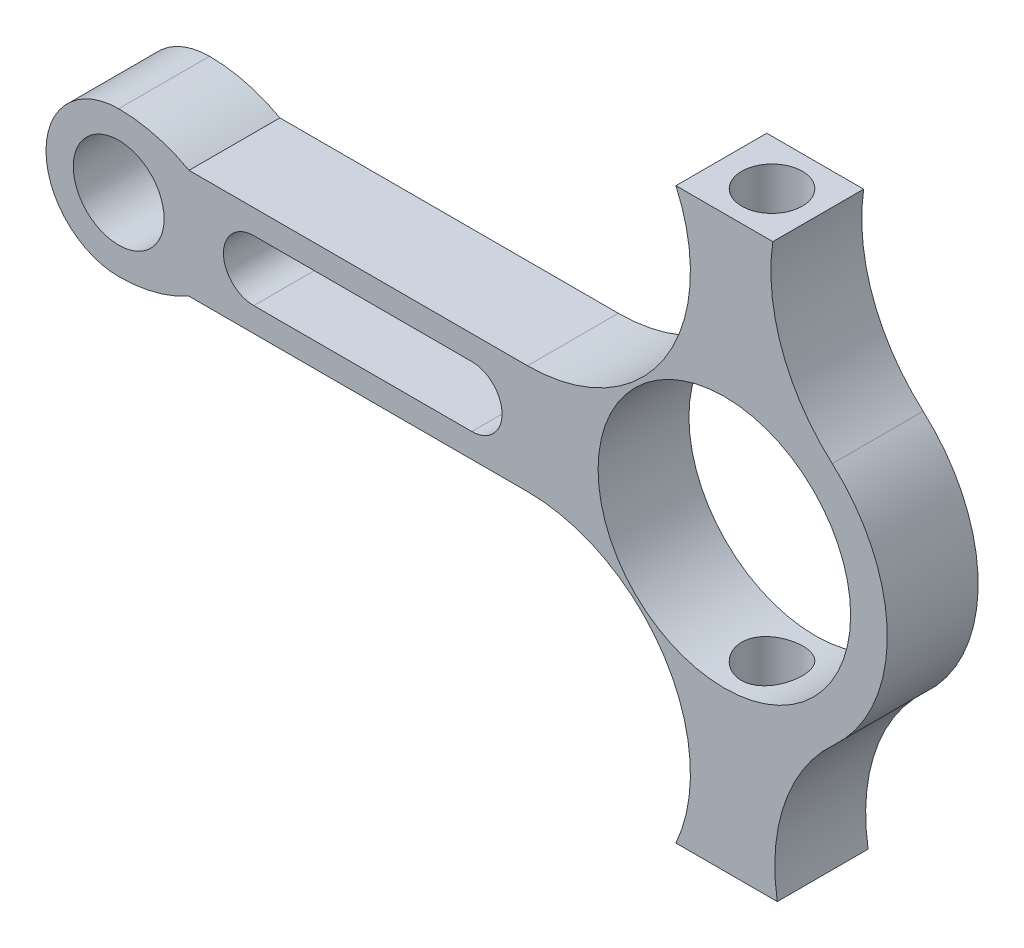
ISO-10303-21;
HEADER;
FILE_DESCRIPTION(('STEP AP214'),'2;1');
FILE_NAME('part.step','',(''),(''),'','','');
FILE_SCHEMA(('AUTOMOTIVE_DESIGN { 1 0 10303 214 1 1 1 1 }'));
ENDSEC;
DATA;
#1=APPLICATION_CONTEXT('core data for automotive mechanical design processes');
#2=APPLICATION_PROTOCOL_DEFINITION('international standard','automotive_design',2000,#1);
#3=PRODUCT_CONTEXT('',#1,'mechanical');
#4=PRODUCT('Part','Part','',(#3));
#5=PRODUCT_RELATED_PRODUCT_CATEGORY('part','',(#4));
#6=PRODUCT_DEFINITION_FORMATION('','',#4);
#7=PRODUCT_DEFINITION_CONTEXT('part definition',#1,'design');
#8=PRODUCT_DEFINITION('design','',#6,#7);
#9=PRODUCT_DEFINITION_SHAPE('','',#8);
#10=(LENGTH_UNIT() NAMED_UNIT(*) SI_UNIT(.MILLI.,.METRE.));
#11=(NAMED_UNIT(*) PLANE_ANGLE_UNIT() SI_UNIT($,.RADIAN.));
#12=(NAMED_UNIT(*) SI_UNIT($,.STERADIAN.) SOLID_ANGLE_UNIT());
#13=UNCERTAINTY_MEASURE_WITH_UNIT(LENGTH_MEASURE(1.E-05),#10,'distance_accuracy_value','');
#14=(GEOMETRIC_REPRESENTATION_CONTEXT(3) GLOBAL_UNCERTAINTY_ASSIGNED_CONTEXT((#13)) GLOBAL_UNIT_ASSIGNED_CONTEXT((#10,
#11,#12)) REPRESENTATION_CONTEXT('',''));
#15=CARTESIAN_POINT('',(0.,0.,0.));
#16=DIRECTION('',(0.,0.,1.));
#17=DIRECTION('',(1.,0.,0.));
#18=AXIS2_PLACEMENT_3D('',#15,#16,#17);
#19=CARTESIAN_POINT('',(137.680790343127,42.6352910054251,15.));
#20=DIRECTION('',(0.,0.,1.));
#21=DIRECTION('',(1.,0.,0.));
#22=AXIS2_PLACEMENT_3D('',#19,#20,#21);
#23=PLANE('',#22);
#24=CARTESIAN_POINT('',(0.,0.,15.));
#25=DIRECTION('',(0.,0.,1.));
#26=DIRECTION('',(1.,0.,0.));
#27=AXIS2_PLACEMENT_3D('',#24,#25,#26);
#28=CIRCLE('',#27,7.5);
#29=CARTESIAN_POINT('',(7.5,0.,15.));
#30=VERTEX_POINT('',#29);
#31=EDGE_CURVE('E208',#30,#30,#28,.T.);
#32=ORIENTED_EDGE('',*,*,#31,.F.);
#33=EDGE_LOOP('',(#32));
#34=FACE_BOUND('',#33,.T.);
#35=DIRECTION('',(-1.,0.,0.));
#36=VECTOR('',#35,1.);
#37=CARTESIAN_POINT('',(100.,47.,15.));
#38=LINE('',#37,#36);
#39=CARTESIAN_POINT('',(108.,47.,15.));
#40=VERTEX_POINT('',#39);
#41=CARTESIAN_POINT('',(92.,47.,15.));
#42=VERTEX_POINT('',#41);
#43=EDGE_CURVE('E212',#40,#42,#38,.T.);
#44=ORIENTED_EDGE('',*,*,#43,.T.);
#45=CARTESIAN_POINT('',(67.4969389667332,35.9,15.));
#46=DIRECTION('',(0.,0.,-1.));
#47=DIRECTION('',(-1.,0.,0.));
#48=AXIS2_PLACEMENT_3D('',#45,#46,#47);
#49=CIRCLE('',#48,26.9);
#50=CARTESIAN_POINT('',(67.4969389667332,9.,15.));
#51=VERTEX_POINT('',#50);
#52=EDGE_CURVE('E216',#42,#51,#49,.T.);
#53=ORIENTED_EDGE('',*,*,#52,.T.);
#54=DIRECTION('',(-1.,0.,0.));
#55=VECTOR('',#54,1.);
#56=CARTESIAN_POINT('',(11.6189500386222,9.,15.));
#57=LINE('',#56,#55);
#58=CARTESIAN_POINT('',(11.6189500386222,9.,15.));
#59=VERTEX_POINT('',#58);
#60=EDGE_CURVE('E218',#51,#59,#57,.T.);
#61=ORIENTED_EDGE('',*,*,#60,.T.);
#62=CARTESIAN_POINT('',(0.,-12.,15.));
#63=DIRECTION('',(0.,0.,1.));
#64=DIRECTION('',(-1.,0.,0.));
#65=AXIS2_PLACEMENT_3D('',#62,#63,#64);
#66=CIRCLE('',#65,24.);
#67=CARTESIAN_POINT('',(0.,12.,15.));
#68=VERTEX_POINT('',#67);
#69=EDGE_CURVE('E222',#59,#68,#66,.T.);
#70=ORIENTED_EDGE('',*,*,#69,.T.);
#71=CARTESIAN_POINT('',(0.,0.,15.));
#72=DIRECTION('',(0.,0.,1.));
#73=DIRECTION('',(1.,0.,0.));
#74=AXIS2_PLACEMENT_3D('',#71,#72,#73);
#75=CIRCLE('',#74,12.);
#76=CARTESIAN_POINT('',(0.,-12.,15.));
#77=VERTEX_POINT('',#76);
#78=EDGE_CURVE('E224',#68,#77,#75,.T.);
#79=ORIENTED_EDGE('',*,*,#78,.T.);
#80=CARTESIAN_POINT('',(0.,12.,15.));
#81=DIRECTION('',(0.,0.,1.));
#82=DIRECTION('',(1.,0.,0.));
#83=AXIS2_PLACEMENT_3D('',#80,#81,#82);
#84=CIRCLE('',#83,24.);
#85=CARTESIAN_POINT('',(11.6189500386223,-9.,15.));
#86=VERTEX_POINT('',#85);
#87=EDGE_CURVE('E223',#77,#86,#84,.T.);
#88=ORIENTED_EDGE('',*,*,#87,.T.);
#89=DIRECTION('',(1.,0.,0.));
#90=VECTOR('',#89,1.);
#91=CARTESIAN_POINT('',(11.6189500386223,-9.,15.));
#92=LINE('',#91,#90);
#93=CARTESIAN_POINT('',(67.4969389667332,-8.99999999999999,15.));
#94=VERTEX_POINT('',#93);
#95=EDGE_CURVE('E226',#86,#94,#92,.T.);
#96=ORIENTED_EDGE('',*,*,#95,.T.);
#97=CARTESIAN_POINT('',(67.4969389667332,-35.9,15.));
#98=DIRECTION('',(0.,0.,-1.));
#99=DIRECTION('',(1.,0.,0.));
#100=AXIS2_PLACEMENT_3D('',#97,#98,#99);
#101=CIRCLE('',#100,26.9);
#102=CARTESIAN_POINT('',(92.,-47.,15.));
#103=VERTEX_POINT('',#102);
#104=EDGE_CURVE('E228',#94,#103,#101,.T.);
#105=ORIENTED_EDGE('',*,*,#104,.T.);
#106=DIRECTION('',(1.,0.,0.));
#107=VECTOR('',#106,1.);
#108=CARTESIAN_POINT('',(100.,-47.,15.));
#109=LINE('',#108,#107);
#110=CARTESIAN_POINT('',(108.73655717955,-47.,15.));
#111=VERTEX_POINT('',#110);
#112=EDGE_CURVE('E233',#103,#111,#109,.T.);
#113=ORIENTED_EDGE('',*,*,#112,.T.);
#114=CARTESIAN_POINT('',(138.32635427095,-42.0559219171047,15.));
#115=DIRECTION('',(0.,0.,-1.));
#116=DIRECTION('',(-1.,0.,0.));
#117=AXIS2_PLACEMENT_3D('',#114,#115,#116);
#118=CIRCLE('',#117,30.);
#119=CARTESIAN_POINT('',(118.119137607883,-19.8823251242551,15.));
#120=VERTEX_POINT('',#119);
#121=EDGE_CURVE('E231',#111,#120,#118,.T.);
#122=ORIENTED_EDGE('',*,*,#121,.T.);
#123=CARTESIAN_POINT('',(100.,0.,15.));
#124=DIRECTION('',(0.,0.,1.));
#125=DIRECTION('',(1.,0.,0.));
#126=AXIS2_PLACEMENT_3D('',#123,#124,#125);
#127=CIRCLE('',#126,26.9);
#128=CARTESIAN_POINT('',(117.813941304572,20.1562272064312,15.));
#129=VERTEX_POINT('',#128);
#130=EDGE_CURVE('E234',#120,#129,#127,.T.);
#131=ORIENTED_EDGE('',*,*,#130,.T.);
#132=CARTESIAN_POINT('',(137.680790343127,42.6352910054251,15.));
#133=DIRECTION('',(0.,0.,-1.));
#134=DIRECTION('',(1.,0.,0.));
#135=AXIS2_PLACEMENT_3D('',#132,#133,#134);
#136=CIRCLE('',#135,30.);
#137=EDGE_CURVE('E240',#129,#40,#136,.T.);
#138=ORIENTED_EDGE('',*,*,#137,.T.);
#139=EDGE_LOOP('',(#44,#53,#61,#70,#79,#88,#96,#105,#113,#122,#131,#138));
#140=FACE_BOUND('',#139,.T.);
#141=CARTESIAN_POINT('',(100.,0.,15.));
#142=DIRECTION('',(0.,0.,1.));
#143=DIRECTION('',(1.,0.,0.));
#144=AXIS2_PLACEMENT_3D('',#141,#142,#143);
#145=CIRCLE('',#144,20.85);
#146=CARTESIAN_POINT('',(120.85,0.,15.));
#147=VERTEX_POINT('',#146);
#148=EDGE_CURVE('E205',#147,#147,#145,.T.);
#149=ORIENTED_EDGE('',*,*,#148,.F.);
#150=EDGE_LOOP('',(#149));
#151=FACE_BOUND('',#150,.T.);
#152=DIRECTION('',(1.,0.,0.));
#153=VECTOR('',#152,1.);
#154=CARTESIAN_POINT('',(22.3,-5.,15.));
#155=LINE('',#154,#153);
#156=CARTESIAN_POINT('',(22.3,-5.,15.));
#157=VERTEX_POINT('',#156);
#158=CARTESIAN_POINT('',(58.3,-5.,15.));
#159=VERTEX_POINT('',#158);
#160=EDGE_CURVE('E175',#157,#159,#155,.T.);
#161=ORIENTED_EDGE('',*,*,#160,.F.);
#162=CARTESIAN_POINT('',(22.3,0.,15.));
#163=DIRECTION('',(0.,0.,1.));
#164=DIRECTION('',(1.,0.,0.));
#165=AXIS2_PLACEMENT_3D('',#162,#163,#164);
#166=CIRCLE('',#165,5.);
#167=CARTESIAN_POINT('',(22.3,5.,15.));
#168=VERTEX_POINT('',#167);
#169=EDGE_CURVE('E164',#168,#157,#166,.T.);
#170=ORIENTED_EDGE('',*,*,#169,.F.);
#171=DIRECTION('',(-1.,0.,0.));
#172=VECTOR('',#171,1.);
#173=CARTESIAN_POINT('',(22.3,5.,15.));
#174=LINE('',#173,#172);
#175=CARTESIAN_POINT('',(58.3,5.,15.));
#176=VERTEX_POINT('',#175);
#177=EDGE_CURVE('E186',#176,#168,#174,.T.);
#178=ORIENTED_EDGE('',*,*,#177,.F.);
#179=CARTESIAN_POINT('',(58.3,0.,15.));
#180=DIRECTION('',(0.,0.,1.));
#181=DIRECTION('',(1.,0.,0.));
#182=AXIS2_PLACEMENT_3D('',#179,#180,#181);
#183=CIRCLE('',#182,5.);
#184=EDGE_CURVE('E183',#159,#176,#183,.T.);
#185=ORIENTED_EDGE('',*,*,#184,.F.);
#186=EDGE_LOOP('',(#161,#170,#178,#185));
#187=FACE_BOUND('',#186,.T.);
#188=ADVANCED_FACE('F44',(#34,#140,#151,#187),#23,.T.);
#189=CARTESIAN_POINT('',(137.680790343127,42.6352910054251,0.));
#190=DIRECTION('',(0.,0.,1.));
#191=DIRECTION('',(1.,0.,0.));
#192=AXIS2_PLACEMENT_3D('',#189,#190,#191);
#193=PLANE('',#192);
#194=CARTESIAN_POINT('',(100.,0.,0.));
#195=DIRECTION('',(0.,0.,1.));
#196=DIRECTION('',(1.,0.,0.));
#197=AXIS2_PLACEMENT_3D('',#194,#195,#196);
#198=CIRCLE('',#197,20.85);
#199=CARTESIAN_POINT('',(120.85,0.,0.));
#200=VERTEX_POINT('',#199);
#201=EDGE_CURVE('E182',#200,#200,#198,.T.);
#202=ORIENTED_EDGE('',*,*,#201,.T.);
#203=EDGE_LOOP('',(#202));
#204=FACE_BOUND('',#203,.T.);
#205=CARTESIAN_POINT('',(0.,0.,0.));
#206=DIRECTION('',(0.,0.,1.));
#207=DIRECTION('',(1.,0.,0.));
#208=AXIS2_PLACEMENT_3D('',#205,#206,#207);
#209=CIRCLE('',#208,7.5);
#210=CARTESIAN_POINT('',(7.5,0.,0.));
#211=VERTEX_POINT('',#210);
#212=EDGE_CURVE('E202',#211,#211,#209,.T.);
#213=ORIENTED_EDGE('',*,*,#212,.T.);
#214=EDGE_LOOP('',(#213));
#215=FACE_BOUND('',#214,.T.);
#216=DIRECTION('',(-1.,0.,0.));
#217=VECTOR('',#216,1.);
#218=CARTESIAN_POINT('',(100.,47.,0.));
#219=LINE('',#218,#217);
#220=CARTESIAN_POINT('',(108.,47.,0.));
#221=VERTEX_POINT('',#220);
#222=CARTESIAN_POINT('',(92.,47.,0.));
#223=VERTEX_POINT('',#222);
#224=EDGE_CURVE('E211',#221,#223,#219,.T.);
#225=ORIENTED_EDGE('',*,*,#224,.F.);
#226=CARTESIAN_POINT('',(137.680790343127,42.6352910054251,0.));
#227=DIRECTION('',(0.,0.,-1.));
#228=DIRECTION('',(1.,0.,0.));
#229=AXIS2_PLACEMENT_3D('',#226,#227,#228);
#230=CIRCLE('',#229,30.);
#231=CARTESIAN_POINT('',(117.813941304572,20.1562272064312,0.));
#232=VERTEX_POINT('',#231);
#233=EDGE_CURVE('E220',#232,#221,#230,.T.);
#234=ORIENTED_EDGE('',*,*,#233,.F.);
#235=CARTESIAN_POINT('',(100.,0.,0.));
#236=DIRECTION('',(0.,0.,1.));
#237=DIRECTION('',(1.,0.,0.));
#238=AXIS2_PLACEMENT_3D('',#235,#236,#237);
#239=CIRCLE('',#238,26.9);
#240=CARTESIAN_POINT('',(118.119137607883,-19.8823251242551,0.));
#241=VERTEX_POINT('',#240);
#242=EDGE_CURVE('E257',#241,#232,#239,.T.);
#243=ORIENTED_EDGE('',*,*,#242,.F.);
#244=CARTESIAN_POINT('',(138.32635427095,-42.0559219171047,0.));
#245=DIRECTION('',(0.,0.,-1.));
#246=DIRECTION('',(-1.,0.,0.));
#247=AXIS2_PLACEMENT_3D('',#244,#245,#246);
#248=CIRCLE('',#247,30.);
#249=CARTESIAN_POINT('',(108.73655717955,-47.,0.));
#250=VERTEX_POINT('',#249);
#251=EDGE_CURVE('E256',#250,#241,#248,.T.);
#252=ORIENTED_EDGE('',*,*,#251,.F.);
#253=DIRECTION('',(1.,0.,0.));
#254=VECTOR('',#253,1.);
#255=CARTESIAN_POINT('',(100.,-47.,0.));
#256=LINE('',#255,#254);
#257=CARTESIAN_POINT('',(92.,-47.,0.));
#258=VERTEX_POINT('',#257);
#259=EDGE_CURVE('E258',#258,#250,#256,.T.);
#260=ORIENTED_EDGE('',*,*,#259,.F.);
#261=CARTESIAN_POINT('',(67.4969389667332,-35.9,0.));
#262=DIRECTION('',(0.,0.,-1.));
#263=DIRECTION('',(1.,0.,0.));
#264=AXIS2_PLACEMENT_3D('',#261,#262,#263);
#265=CIRCLE('',#264,26.9);
#266=CARTESIAN_POINT('',(67.4969389667332,-8.99999999999999,0.));
#267=VERTEX_POINT('',#266);
#268=EDGE_CURVE('E251',#267,#258,#265,.T.);
#269=ORIENTED_EDGE('',*,*,#268,.F.);
#270=DIRECTION('',(1.,0.,0.));
#271=VECTOR('',#270,1.);
#272=CARTESIAN_POINT('',(11.6189500386223,-9.,0.));
#273=LINE('',#272,#271);
#274=CARTESIAN_POINT('',(11.6189500386223,-9.,0.));
#275=VERTEX_POINT('',#274);
#276=EDGE_CURVE('E253',#275,#267,#273,.T.);
#277=ORIENTED_EDGE('',*,*,#276,.F.);
#278=CARTESIAN_POINT('',(0.,12.,0.));
#279=DIRECTION('',(0.,0.,1.));
#280=DIRECTION('',(1.,0.,0.));
#281=AXIS2_PLACEMENT_3D('',#278,#279,#280);
#282=CIRCLE('',#281,24.);
#283=CARTESIAN_POINT('',(0.,-12.,0.));
#284=VERTEX_POINT('',#283);
#285=EDGE_CURVE('E247',#284,#275,#282,.T.);
#286=ORIENTED_EDGE('',*,*,#285,.F.);
#287=CARTESIAN_POINT('',(0.,0.,0.));
#288=DIRECTION('',(0.,0.,1.));
#289=DIRECTION('',(1.,0.,0.));
#290=AXIS2_PLACEMENT_3D('',#287,#288,#289);
#291=CIRCLE('',#290,12.);
#292=CARTESIAN_POINT('',(0.,12.,0.));
#293=VERTEX_POINT('',#292);
#294=EDGE_CURVE('E250',#293,#284,#291,.T.);
#295=ORIENTED_EDGE('',*,*,#294,.F.);
#296=CARTESIAN_POINT('',(0.,-12.,0.));
#297=DIRECTION('',(0.,0.,1.));
#298=DIRECTION('',(-1.,0.,0.));
#299=AXIS2_PLACEMENT_3D('',#296,#297,#298);
#300=CIRCLE('',#299,24.);
#301=CARTESIAN_POINT('',(11.6189500386222,9.,0.));
#302=VERTEX_POINT('',#301);
#303=EDGE_CURVE('E242',#302,#293,#300,.T.);
#304=ORIENTED_EDGE('',*,*,#303,.F.);
#305=DIRECTION('',(-1.,0.,0.));
#306=VECTOR('',#305,1.);
#307=CARTESIAN_POINT('',(11.6189500386222,9.,0.));
#308=LINE('',#307,#306);
#309=CARTESIAN_POINT('',(67.4969389667332,9.,0.));
#310=VERTEX_POINT('',#309);
#311=EDGE_CURVE('E245',#310,#302,#308,.T.);
#312=ORIENTED_EDGE('',*,*,#311,.F.);
#313=CARTESIAN_POINT('',(67.4969389667332,35.9,0.));
#314=DIRECTION('',(0.,0.,-1.));
#315=DIRECTION('',(-1.,0.,0.));
#316=AXIS2_PLACEMENT_3D('',#313,#314,#315);
#317=CIRCLE('',#316,26.9);
#318=EDGE_CURVE('E244',#223,#310,#317,.T.);
#319=ORIENTED_EDGE('',*,*,#318,.F.);
#320=EDGE_LOOP('',(#225,#234,#243,#252,#260,#269,#277,#286,#295,#304,#312,#319));
#321=FACE_BOUND('',#320,.T.);
#322=CARTESIAN_POINT('',(22.3,0.,0.));
#323=DIRECTION('',(0.,0.,1.));
#324=DIRECTION('',(1.,0.,0.));
#325=AXIS2_PLACEMENT_3D('',#322,#323,#324);
#326=CIRCLE('',#325,5.);
#327=CARTESIAN_POINT('',(22.3,5.,0.));
#328=VERTEX_POINT('',#327);
#329=CARTESIAN_POINT('',(22.3,-5.,0.));
#330=VERTEX_POINT('',#329);
#331=EDGE_CURVE('E73',#328,#330,#326,.T.);
#332=ORIENTED_EDGE('',*,*,#331,.T.);
#333=DIRECTION('',(1.,0.,0.));
#334=VECTOR('',#333,1.);
#335=CARTESIAN_POINT('',(22.3,-5.,0.));
#336=LINE('',#335,#334);
#337=CARTESIAN_POINT('',(58.3,-5.,0.));
#338=VERTEX_POINT('',#337);
#339=EDGE_CURVE('E179',#330,#338,#336,.T.);
#340=ORIENTED_EDGE('',*,*,#339,.T.);
#341=CARTESIAN_POINT('',(58.3,0.,0.));
#342=DIRECTION('',(0.,0.,1.));
#343=DIRECTION('',(1.,0.,0.));
#344=AXIS2_PLACEMENT_3D('',#341,#342,#343);
#345=CIRCLE('',#344,5.);
#346=CARTESIAN_POINT('',(58.3,5.,0.));
#347=VERTEX_POINT('',#346);
#348=EDGE_CURVE('E192',#338,#347,#345,.T.);
#349=ORIENTED_EDGE('',*,*,#348,.T.);
#350=DIRECTION('',(-1.,0.,0.));
#351=VECTOR('',#350,1.);
#352=CARTESIAN_POINT('',(22.3,5.,0.));
#353=LINE('',#352,#351);
#354=EDGE_CURVE('E173',#347,#328,#353,.T.);
#355=ORIENTED_EDGE('',*,*,#354,.T.);
#356=EDGE_LOOP('',(#332,#340,#349,#355));
#357=FACE_BOUND('',#356,.T.);
#358=ADVANCED_FACE('F326',(#204,#215,#321,#357),#193,.F.);
#359=CARTESIAN_POINT('',(100.,47.,15.));
#360=DIRECTION('',(0.,-1.,0.));
#361=DIRECTION('',(0.,0.,-1.));
#362=AXIS2_PLACEMENT_3D('',#359,#360,#361);
#363=PLANE('',#362);
#364=CARTESIAN_POINT('',(100.368278589775,47.,7.5));
#365=DIRECTION('',(0.,-1.,0.));
#366=DIRECTION('',(0.,0.,-1.));
#367=AXIS2_PLACEMENT_3D('',#364,#365,#366);
#368=CIRCLE('',#367,5.);
#369=CARTESIAN_POINT('',(100.368278589775,47.,2.5));
#370=VERTEX_POINT('',#369);
#371=EDGE_CURVE('E298',#370,#370,#368,.T.);
#372=ORIENTED_EDGE('',*,*,#371,.T.);
#373=EDGE_LOOP('',(#372));
#374=FACE_BOUND('',#373,.T.);
#375=ORIENTED_EDGE('',*,*,#224,.T.);
#376=DIRECTION('',(0.,0.,-1.));
#377=VECTOR('',#376,1.);
#378=CARTESIAN_POINT('',(92.,47.,15.));
#379=LINE('',#378,#377);
#380=EDGE_CURVE('E11',#42,#223,#379,.T.);
#381=ORIENTED_EDGE('',*,*,#380,.F.);
#382=ORIENTED_EDGE('',*,*,#43,.F.);
#383=DIRECTION('',(0.,0.,-1.));
#384=VECTOR('',#383,1.);
#385=CARTESIAN_POINT('',(108.,47.,15.));
#386=LINE('',#385,#384);
#387=EDGE_CURVE('E239',#40,#221,#386,.T.);
#388=ORIENTED_EDGE('',*,*,#387,.T.);
#389=EDGE_LOOP('',(#375,#381,#382,#388));
#390=FACE_BOUND('',#389,.T.);
#391=ADVANCED_FACE('F50',(#374,#390),#363,.F.);
#392=CARTESIAN_POINT('',(67.4969389667332,35.9,15.));
#393=DIRECTION('',(0.,0.,-1.));
#394=DIRECTION('',(-1.,0.,0.));
#395=AXIS2_PLACEMENT_3D('',#392,#393,#394);
#396=CYLINDRICAL_SURFACE('',#395,26.9);
#397=ORIENTED_EDGE('',*,*,#318,.T.);
#398=DIRECTION('',(0.,0.,-1.));
#399=VECTOR('',#398,1.);
#400=CARTESIAN_POINT('',(67.4969389667332,9.,15.));
#401=LINE('',#400,#399);
#402=EDGE_CURVE('E56',#51,#310,#401,.T.);
#403=ORIENTED_EDGE('',*,*,#402,.F.);
#404=ORIENTED_EDGE('',*,*,#52,.F.);
#405=ORIENTED_EDGE('',*,*,#380,.T.);
#406=EDGE_LOOP('',(#397,#403,#404,#405));
#407=FACE_BOUND('',#406,.T.);
#408=ADVANCED_FACE('F376',(#407),#396,.F.);
#409=CARTESIAN_POINT('',(11.6189500386222,9.,15.));
#410=DIRECTION('',(0.,-1.,0.));
#411=DIRECTION('',(0.,0.,-1.));
#412=AXIS2_PLACEMENT_3D('',#409,#410,#411);
#413=PLANE('',#412);
#414=ORIENTED_EDGE('',*,*,#311,.T.);
#415=DIRECTION('',(0.,0.,-1.));
#416=VECTOR('',#415,1.);
#417=CARTESIAN_POINT('',(11.6189500386222,9.,15.));
#418=LINE('',#417,#416);
#419=EDGE_CURVE('E289',#59,#302,#418,.T.);
#420=ORIENTED_EDGE('',*,*,#419,.F.);
#421=ORIENTED_EDGE('',*,*,#60,.F.);
#422=ORIENTED_EDGE('',*,*,#402,.T.);
#423=EDGE_LOOP('',(#414,#420,#421,#422));
#424=FACE_BOUND('',#423,.T.);
#425=ADVANCED_FACE('F373',(#424),#413,.F.);
#426=CARTESIAN_POINT('',(0.,-12.,15.));
#427=DIRECTION('',(0.,0.,-1.));
#428=DIRECTION('',(-1.,0.,0.));
#429=AXIS2_PLACEMENT_3D('',#426,#427,#428);
#430=CYLINDRICAL_SURFACE('',#429,24.);
#431=ORIENTED_EDGE('',*,*,#303,.T.);
#432=DIRECTION('',(0.,0.,-1.));
#433=VECTOR('',#432,1.);
#434=CARTESIAN_POINT('',(0.,12.,15.));
#435=LINE('',#434,#433);
#436=EDGE_CURVE('E290',#68,#293,#435,.T.);
#437=ORIENTED_EDGE('',*,*,#436,.F.);
#438=ORIENTED_EDGE('',*,*,#69,.F.);
#439=ORIENTED_EDGE('',*,*,#419,.T.);
#440=EDGE_LOOP('',(#431,#437,#438,#439));
#441=FACE_BOUND('',#440,.T.);
#442=ADVANCED_FACE('F369',(#441),#430,.T.);
#443=CARTESIAN_POINT('',(0.,0.,15.));
#444=DIRECTION('',(0.,0.,-1.));
#445=DIRECTION('',(-1.,0.,0.));
#446=AXIS2_PLACEMENT_3D('',#443,#444,#445);
#447=CYLINDRICAL_SURFACE('',#446,12.);
#448=ORIENTED_EDGE('',*,*,#294,.T.);
#449=DIRECTION('',(0.,0.,-1.));
#450=VECTOR('',#449,1.);
#451=CARTESIAN_POINT('',(0.,-12.,15.));
#452=LINE('',#451,#450);
#453=EDGE_CURVE('E283',#77,#284,#452,.T.);
#454=ORIENTED_EDGE('',*,*,#453,.F.);
#455=ORIENTED_EDGE('',*,*,#78,.F.);
#456=ORIENTED_EDGE('',*,*,#436,.T.);
#457=EDGE_LOOP('',(#448,#454,#455,#456));
#458=FACE_BOUND('',#457,.T.);
#459=ADVANCED_FACE('F364',(#458),#447,.T.);
#460=CARTESIAN_POINT('',(0.,12.,15.));
#461=DIRECTION('',(0.,0.,-1.));
#462=DIRECTION('',(-1.,0.,0.));
#463=AXIS2_PLACEMENT_3D('',#460,#461,#462);
#464=CYLINDRICAL_SURFACE('',#463,24.);
#465=ORIENTED_EDGE('',*,*,#285,.T.);
#466=DIRECTION('',(0.,0.,-1.));
#467=VECTOR('',#466,1.);
#468=CARTESIAN_POINT('',(11.6189500386223,-9.,15.));
#469=LINE('',#468,#467);
#470=EDGE_CURVE('E284',#86,#275,#469,.T.);
#471=ORIENTED_EDGE('',*,*,#470,.F.);
#472=ORIENTED_EDGE('',*,*,#87,.F.);
#473=ORIENTED_EDGE('',*,*,#453,.T.);
#474=EDGE_LOOP('',(#465,#471,#472,#473));
#475=FACE_BOUND('',#474,.T.);
#476=ADVANCED_FACE('F363',(#475),#464,.T.);
#477=CARTESIAN_POINT('',(11.6189500386223,-9.,15.));
#478=DIRECTION('',(0.,1.,0.));
#479=DIRECTION('',(-1.,0.,0.));
#480=AXIS2_PLACEMENT_3D('',#477,#478,#479);
#481=PLANE('',#480);
#482=ORIENTED_EDGE('',*,*,#276,.T.);
#483=DIRECTION('',(0.,0.,-1.));
#484=VECTOR('',#483,1.);
#485=CARTESIAN_POINT('',(67.4969389667332,-8.99999999999999,15.));
#486=LINE('',#485,#484);
#487=EDGE_CURVE('E279',#94,#267,#486,.T.);
#488=ORIENTED_EDGE('',*,*,#487,.F.);
#489=ORIENTED_EDGE('',*,*,#95,.F.);
#490=ORIENTED_EDGE('',*,*,#470,.T.);
#491=EDGE_LOOP('',(#482,#488,#489,#490));
#492=FACE_BOUND('',#491,.T.);
#493=ADVANCED_FACE('F360',(#492),#481,.F.);
#494=CARTESIAN_POINT('',(67.4969389667332,-35.9,15.));
#495=DIRECTION('',(0.,0.,-1.));
#496=DIRECTION('',(-1.,0.,0.));
#497=AXIS2_PLACEMENT_3D('',#494,#495,#496);
#498=CYLINDRICAL_SURFACE('',#497,26.9);
#499=ORIENTED_EDGE('',*,*,#268,.T.);
#500=DIRECTION('',(0.,0.,-1.));
#501=VECTOR('',#500,1.);
#502=CARTESIAN_POINT('',(92.,-47.,15.));
#503=LINE('',#502,#501);
#504=EDGE_CURVE('E274',#103,#258,#503,.T.);
#505=ORIENTED_EDGE('',*,*,#504,.F.);
#506=ORIENTED_EDGE('',*,*,#104,.F.);
#507=ORIENTED_EDGE('',*,*,#487,.T.);
#508=EDGE_LOOP('',(#499,#505,#506,#507));
#509=FACE_BOUND('',#508,.T.);
#510=ADVANCED_FACE('F355',(#509),#498,.F.);
#511=CARTESIAN_POINT('',(100.,-47.,15.));
#512=DIRECTION('',(0.,1.,0.));
#513=DIRECTION('',(0.,0.,1.));
#514=AXIS2_PLACEMENT_3D('',#511,#512,#513);
#515=PLANE('',#514);
#516=CARTESIAN_POINT('',(100.368278589775,-47.,7.5));
#517=DIRECTION('',(0.,-1.,0.));
#518=DIRECTION('',(0.,0.,-1.));
#519=AXIS2_PLACEMENT_3D('',#516,#517,#518);
#520=CIRCLE('',#519,5.);
#521=CARTESIAN_POINT('',(100.368278589775,-47.,2.5));
#522=VERTEX_POINT('',#521);
#523=EDGE_CURVE('E675',#522,#522,#520,.T.);
#524=ORIENTED_EDGE('',*,*,#523,.F.);
#525=EDGE_LOOP('',(#524));
#526=FACE_BOUND('',#525,.T.);
#527=ORIENTED_EDGE('',*,*,#259,.T.);
#528=DIRECTION('',(0.,0.,-1.));
#529=VECTOR('',#528,1.);
#530=CARTESIAN_POINT('',(108.73655717955,-47.,15.));
#531=LINE('',#530,#529);
#532=EDGE_CURVE('E275',#111,#250,#531,.T.);
#533=ORIENTED_EDGE('',*,*,#532,.F.);
#534=ORIENTED_EDGE('',*,*,#112,.F.);
#535=ORIENTED_EDGE('',*,*,#504,.T.);
#536=EDGE_LOOP('',(#527,#533,#534,#535));
#537=FACE_BOUND('',#536,.T.);
#538=ADVANCED_FACE('F349',(#526,#537),#515,.F.);
#539=CARTESIAN_POINT('',(138.32635427095,-42.0559219171047,15.));
#540=DIRECTION('',(0.,0.,-1.));
#541=DIRECTION('',(-1.,0.,0.));
#542=AXIS2_PLACEMENT_3D('',#539,#540,#541);
#543=CYLINDRICAL_SURFACE('',#542,30.);
#544=ORIENTED_EDGE('',*,*,#251,.T.);
#545=DIRECTION('',(0.,0.,-1.));
#546=VECTOR('',#545,1.);
#547=CARTESIAN_POINT('',(118.119137607883,-19.8823251242551,15.));
#548=LINE('',#547,#546);
#549=EDGE_CURVE('E267',#120,#241,#548,.T.);
#550=ORIENTED_EDGE('',*,*,#549,.F.);
#551=ORIENTED_EDGE('',*,*,#121,.F.);
#552=ORIENTED_EDGE('',*,*,#532,.T.);
#553=EDGE_LOOP('',(#544,#550,#551,#552));
#554=FACE_BOUND('',#553,.T.);
#555=ADVANCED_FACE('F344',(#554),#543,.F.);
#556=CARTESIAN_POINT('',(100.,0.,15.));
#557=DIRECTION('',(0.,0.,-1.));
#558=DIRECTION('',(-1.,0.,0.));
#559=AXIS2_PLACEMENT_3D('',#556,#557,#558);
#560=CYLINDRICAL_SURFACE('',#559,26.9);
#561=ORIENTED_EDGE('',*,*,#242,.T.);
#562=DIRECTION('',(0.,0.,-1.));
#563=VECTOR('',#562,1.);
#564=CARTESIAN_POINT('',(117.813941304572,20.1562272064312,15.));
#565=LINE('',#564,#563);
#566=EDGE_CURVE('E266',#129,#232,#565,.T.);
#567=ORIENTED_EDGE('',*,*,#566,.F.);
#568=ORIENTED_EDGE('',*,*,#130,.F.);
#569=ORIENTED_EDGE('',*,*,#549,.T.);
#570=EDGE_LOOP('',(#561,#567,#568,#569));
#571=FACE_BOUND('',#570,.T.);
#572=ADVANCED_FACE('F343',(#571),#560,.T.);
#573=CARTESIAN_POINT('',(137.680790343127,42.6352910054251,15.));
#574=DIRECTION('',(0.,0.,-1.));
#575=DIRECTION('',(-1.,0.,0.));
#576=AXIS2_PLACEMENT_3D('',#573,#574,#575);
#577=CYLINDRICAL_SURFACE('',#576,30.);
#578=ORIENTED_EDGE('',*,*,#233,.T.);
#579=ORIENTED_EDGE('',*,*,#387,.F.);
#580=ORIENTED_EDGE('',*,*,#137,.F.);
#581=ORIENTED_EDGE('',*,*,#566,.T.);
#582=EDGE_LOOP('',(#578,#579,#580,#581));
#583=FACE_BOUND('',#582,.T.);
#584=ADVANCED_FACE('F340',(#583),#577,.F.);
#585=CARTESIAN_POINT('',(0.,0.,15.));
#586=DIRECTION('',(0.,0.,-1.));
#587=DIRECTION('',(-1.,0.,0.));
#588=AXIS2_PLACEMENT_3D('',#585,#586,#587);
#589=CYLINDRICAL_SURFACE('',#588,7.5);
#590=ORIENTED_EDGE('',*,*,#31,.T.);
#591=EDGE_LOOP('',(#590));
#592=FACE_BOUND('',#591,.T.);
#593=ORIENTED_EDGE('',*,*,#212,.F.);
#594=EDGE_LOOP('',(#593));
#595=FACE_BOUND('',#594,.T.);
#596=ADVANCED_FACE('F323',(#592,#595),#589,.F.);
#597=CARTESIAN_POINT('',(100.,0.,15.));
#598=DIRECTION('',(0.,0.,-1.));
#599=DIRECTION('',(-1.,0.,0.));
#600=AXIS2_PLACEMENT_3D('',#597,#598,#599);
#601=CYLINDRICAL_SURFACE('',#600,20.85);
#602=CARTESIAN_POINT('',(100.368278589775,20.8467472493987,2.5));
#603=CARTESIAN_POINT('',(100.645623782383,20.8418425276496,2.50000873074007));
#604=CARTESIAN_POINT('',(100.922971019068,20.8313557012789,2.52315448487608));
#605=CARTESIAN_POINT('',(101.469538630426,20.7999534036774,2.61490749386963));
#606=CARTESIAN_POINT('',(101.738753494642,20.7790310223325,2.68354488184995));
#607=CARTESIAN_POINT('',(102.261093036554,20.7286938941873,2.86389235775413));
#608=CARTESIAN_POINT('',(102.514237591091,20.6992898979575,2.97554797920609));
#609=CARTESIAN_POINT('',(102.99813006646,20.6347614739051,3.23857504242802));
#610=CARTESIAN_POINT('',(103.228877738837,20.5996369826349,3.38994692471311));
#611=CARTESIAN_POINT('',(103.666239315637,20.5263569870843,3.73146395318609));
#612=CARTESIAN_POINT('',(103.872320453945,20.4881570449738,3.92228200869241));
#613=CARTESIAN_POINT('',(104.249840250739,20.4131938560214,4.33584432210659));
#614=CARTESIAN_POINT('',(104.421275309141,20.3764307588023,4.55859189371271));
#615=CARTESIAN_POINT('',(104.726597097053,20.3077975858423,5.03310087520545));
#616=CARTESIAN_POINT('',(104.860005591879,20.2759919317506,5.28518005999728));
#617=CARTESIAN_POINT('',(105.082305669924,20.2214209100405,5.8091712371062));
#618=CARTESIAN_POINT('',(105.171205243867,20.1986539198551,6.08107965941346));
#619=CARTESIAN_POINT('',(105.299973030523,20.1652461138782,6.63042857560054));
#620=CARTESIAN_POINT('',(105.340913677225,20.1543404759228,6.90760129726517));
#621=CARTESIAN_POINT('',(105.375947604529,20.145025328736,7.46507897829386));
#622=CARTESIAN_POINT('',(105.370048745884,20.1466137227163,7.74538340420091));
#623=CARTESIAN_POINT('',(105.312374493529,20.1618945240154,8.29374878706753));
#624=CARTESIAN_POINT('',(105.261750762522,20.1752830578781,8.56194059956306));
#625=CARTESIAN_POINT('',(105.117886994795,20.2122536356695,9.08588812848482));
#626=CARTESIAN_POINT('',(105.024643914446,20.2358364076054,9.34164295528997));
#627=CARTESIAN_POINT('',(104.797171414288,20.2909688410816,9.83664535020806));
#628=CARTESIAN_POINT('',(104.662510731523,20.3226016960477,10.0756850989969));
#629=CARTESIAN_POINT('',(104.35636150071,20.3904176424941,10.5281758359783));
#630=CARTESIAN_POINT('',(104.184866307381,20.4266015545378,10.741622196049));
#631=CARTESIAN_POINT('',(103.803794426103,20.5010337074574,11.1436564005854));
#632=CARTESIAN_POINT('',(103.593222273319,20.5393112818008,11.3312963739832));
#633=CARTESIAN_POINT('',(103.143228754256,20.6129696702683,11.6687832389196));
#634=CARTESIAN_POINT('',(102.903805944874,20.648350339341,11.8186282388008));
#635=CARTESIAN_POINT('',(102.400910309918,20.7128632163755,12.076984464168));
#636=CARTESIAN_POINT('',(102.137299562139,20.7419559523609,12.1852377204259));
#637=CARTESIAN_POINT('',(101.594737081053,20.7907047202026,12.355574760462));
#638=CARTESIAN_POINT('',(101.315788086816,20.8103624308831,12.417666759038));
#639=CARTESIAN_POINT('',(100.757675860204,20.8380564328646,12.4925667132936));
#640=CARTESIAN_POINT('',(100.478681004653,20.846362316771,12.5065304006547));
#641=CARTESIAN_POINT('',(99.9221660479503,20.8517110397355,12.4878329464588));
#642=CARTESIAN_POINT('',(99.6446457977324,20.8487550398095,12.4551766112942));
#643=CARTESIAN_POINT('',(99.1038453435579,20.8324606862583,12.3452118897285));
#644=CARTESIAN_POINT('',(98.8404037439593,20.8192986417342,12.2686674633288));
#645=CARTESIAN_POINT('',(98.3300273003119,20.7845898730065,12.0738559853888));
#646=CARTESIAN_POINT('',(98.0830937527842,20.7630424911337,11.955585661319));
#647=CARTESIAN_POINT('',(97.6090594970899,20.7138482819378,11.6788803036967));
#648=CARTESIAN_POINT('',(97.3822689453844,20.6861235791889,11.5199282199));
#649=CARTESIAN_POINT('',(96.9581458868137,20.6280276981795,11.1670323679368));
#650=CARTESIAN_POINT('',(96.7608177658692,20.597656126957,10.9730833994362));
#651=CARTESIAN_POINT('',(96.3967548614976,20.5371370177676,10.5506447748149));
#652=CARTESIAN_POINT('',(96.2307884216917,20.5070090997675,10.3214892383113));
#653=CARTESIAN_POINT('',(95.939621220778,20.4513540863041,9.83807628347002));
#654=CARTESIAN_POINT('',(95.8144193875709,20.4258268698512,9.58381952551771));
#655=CARTESIAN_POINT('',(95.6088666660466,20.3826278611197,9.0580181650174));
#656=CARTESIAN_POINT('',(95.5283805836782,20.3649324235228,8.78652846906912));
#657=CARTESIAN_POINT('',(95.4143124126253,20.3395536906632,8.23342805764289));
#658=CARTESIAN_POINT('',(95.3807223675945,20.3318686970511,7.95181906731475));
#659=CARTESIAN_POINT('',(95.3617899570051,20.3275573026932,7.39330070955679));
#660=CARTESIAN_POINT('',(95.3753732601068,20.3306846530343,7.11642915273927));
#661=CARTESIAN_POINT('',(95.4479617496418,20.3470588888266,6.56902673915404));
#662=CARTESIAN_POINT('',(95.5069663294426,20.3603056391262,6.29849579775277));
#663=CARTESIAN_POINT('',(95.668149708827,20.3952022560247,5.7725377263878));
#664=CARTESIAN_POINT('',(95.7701371313532,20.4168148401664,5.51704929905744));
#665=CARTESIAN_POINT('',(96.0142528184888,20.465867943213,5.02664035534603));
#666=CARTESIAN_POINT('',(96.1563857083299,20.4933091335517,4.79172221299248));
#667=CARTESIAN_POINT('',(96.4803012698754,20.5514424176249,4.34379693043272));
#668=CARTESIAN_POINT('',(96.6628549057007,20.5821907410091,4.13135446335142));
#669=CARTESIAN_POINT('',(97.0609301262032,20.6427910739105,3.7397587506064));
#670=CARTESIAN_POINT('',(97.2764586838965,20.672642892248,3.56061256370241));
#671=CARTESIAN_POINT('',(97.7376388995746,20.7282119755348,3.23856623946167));
#672=CARTESIAN_POINT('',(97.9836317680618,20.7538732198641,3.09614445192424));
#673=CARTESIAN_POINT('',(98.49664146444,20.7973183863439,2.85487510121846));
#674=CARTESIAN_POINT('',(98.7636416983147,20.8151084539109,2.75599354433083));
#675=CARTESIAN_POINT('',(99.2535463944993,20.8377625759193,2.6206744761741));
#676=CARTESIAN_POINT('',(99.4739911580778,20.8445521249144,2.5755013841985));
#677=CARTESIAN_POINT('',(99.9190498420359,20.8510303841931,2.51516138891329));
#678=CARTESIAN_POINT('',(100.143663545552,20.8507194628062,2.49999292918853));
#679=CARTESIAN_POINT('',(100.368278589775,20.8467472493987,2.5));
#680=B_SPLINE_CURVE_WITH_KNOTS('',3,(#602,#603,#604,#605,#606,#607,#608,#609,#610,#611,#612,
#613,#614,#615,#616,#617,#618,#619,#620,#621,#622,#623,#624,#625,#626,#627,#628,#629,#630,#631,
#632,#633,#634,#635,#636,#637,#638,#639,#640,#641,#642,#643,#644,#645,#646,#647,#648,#649,#650,
#651,#652,#653,#654,#655,#656,#657,#658,#659,#660,#661,#662,#663,#664,#665,#666,#667,#668,#669,
#670,#671,#672,#673,#674,#675,#676,#677,#678,#679),.UNSPECIFIED.,.T.,.F.,(4,2,2,2,2,2,2,2,2,2,2,
2,2,2,2,2,2,2,2,2,2,2,2,2,2,2,2,2,2,2,2,2,2,2,2,2,2,2,4),(0.,0.831338850420109,1.66322892098789,
2.49406915764265,3.32491860999756,4.17132458424978,5.0178184636043,5.87453055674789,
6.73108878842034,7.56810354197133,8.40497782803863,9.22091099808561,10.0369024464685,
10.8616958484233,11.6866381757889,12.5365477666369,13.3864998874475,14.2416417862737,
15.0966314686994,15.9309410901016,16.765164702755,17.5852896927841,18.4054790188796,
19.23666065018,20.0679658921151,20.9175552644107,21.7671222909057,22.6141065518635,
23.4609470966414,24.2886292873003,25.1163004238849,25.9403247278132,26.764444007822,
27.6058942477496,28.4475226708557,29.2996152739409,30.1510414271952,30.8243572249789,
31.4976380952757),.UNSPECIFIED.);
#681=CARTESIAN_POINT('',(100.368278589775,20.8467472493987,2.5));
#682=VERTEX_POINT('',#681);
#683=EDGE_CURVE('E47',#682,#682,#680,.T.);
#684=ORIENTED_EDGE('',*,*,#683,.F.);
#685=EDGE_LOOP('',(#684));
#686=FACE_BOUND('',#685,.T.);
#687=CARTESIAN_POINT('',(100.368278589775,-20.8467472493987,2.5));
#688=CARTESIAN_POINT('',(100.092337399302,-20.8516173994047,2.50000802601551));
#689=CARTESIAN_POINT('',(99.8162070086057,-20.8509650413589,2.52291927977566));
#690=CARTESIAN_POINT('',(99.2716351275977,-20.8390573644441,2.61393016933857));
#691=CARTESIAN_POINT('',(99.0031981188879,-20.8277959898942,2.68205560706596));
#692=CARTESIAN_POINT('',(98.4819668829425,-20.7963028583024,2.86128277297178));
#693=CARTESIAN_POINT('',(98.2291568818237,-20.7760803208791,2.97234031585905));
#694=CARTESIAN_POINT('',(97.7456874945195,-20.7291979243426,3.23413415789638));
#695=CARTESIAN_POINT('',(97.5150284761665,-20.7025379583573,3.38487111579502));
#696=CARTESIAN_POINT('',(97.0784410473345,-20.6454903087326,3.72447036651447));
#697=CARTESIAN_POINT('',(96.8729485066893,-20.6150515121289,3.91388437238077));
#698=CARTESIAN_POINT('',(96.496282855276,-20.5543899136753,4.32427340082076));
#699=CARTESIAN_POINT('',(96.32511331163,-20.5241671345903,4.54525169972752));
#700=CARTESIAN_POINT('',(96.0195013865961,-20.4671134440966,5.01642892220762));
#701=CARTESIAN_POINT('',(95.8856364808459,-20.4403389853151,5.26700996328333));
#702=CARTESIAN_POINT('',(95.6620525087134,-20.3940636512276,5.78777757188495));
#703=CARTESIAN_POINT('',(95.5723283165995,-20.3745619314563,6.05796185884919));
#704=CARTESIAN_POINT('',(95.4408819131027,-20.3455511485819,6.60611404816982));
#705=CARTESIAN_POINT('',(95.3984785130611,-20.335900456541,6.88391089495843));
#706=CARTESIAN_POINT('',(95.3607682851848,-20.3273320792195,7.44283019465444));
#707=CARTESIAN_POINT('',(95.365455295556,-20.3284129897052,7.72395220765471));
#708=CARTESIAN_POINT('',(95.4211969784882,-20.3410377787272,8.27575834922346));
#709=CARTESIAN_POINT('',(95.4713482625372,-20.3523777967978,8.54653914799617));
#710=CARTESIAN_POINT('',(95.6151512567264,-20.3838408461047,9.07574747914436));
#711=CARTESIAN_POINT('',(95.7088056357658,-20.4039644162041,9.33417425253184));
#712=CARTESIAN_POINT('',(95.9377446395419,-20.4507767703428,9.8337724341134));
#713=CARTESIAN_POINT('',(96.0733612307475,-20.4775175532468,10.0747866339453));
#714=CARTESIAN_POINT('',(96.3821700085184,-20.5343220925102,10.5309790927589));
#715=CARTESIAN_POINT('',(96.5553676024998,-20.5643863267652,10.7461536268211));
#716=CARTESIAN_POINT('',(96.9390400294985,-20.6250210800111,11.1495919537996));
#717=CARTESIAN_POINT('',(97.1502606109422,-20.6555879216793,11.3371478973151));
#718=CARTESIAN_POINT('',(97.6015807285368,-20.712840023951,11.6742924422028));
#719=CARTESIAN_POINT('',(97.841680365964,-20.7395252709414,11.8238809104206));
#720=CARTESIAN_POINT('',(98.3442582379911,-20.7856831650193,12.08071737231));
#721=CARTESIAN_POINT('',(98.6067389744798,-20.8051550044466,12.1879606248235));
#722=CARTESIAN_POINT('',(99.1465304333041,-20.8342758477445,12.3566710643245));
#723=CARTESIAN_POINT('',(99.4238386017573,-20.8439265375138,12.418146107397));
#724=CARTESIAN_POINT('',(99.9785723539058,-20.8517918084599,12.4924590929837));
#725=CARTESIAN_POINT('',(100.255849624449,-20.8502633880853,12.5063793058351));
#726=CARTESIAN_POINT('',(100.808594996448,-20.836148758444,12.4882437399244));
#727=CARTESIAN_POINT('',(101.084063208821,-20.8235632336056,12.4561908067947));
#728=CARTESIAN_POINT('',(101.622575737253,-20.7885036670891,12.3478280150362));
#729=CARTESIAN_POINT('',(101.885716835688,-20.7661299015309,12.2719645171766));
#730=CARTESIAN_POINT('',(102.395449640506,-20.713523106036,12.0787437415365));
#731=CARTESIAN_POINT('',(102.642039464606,-20.6832891841063,11.961381753845));
#732=CARTESIAN_POINT('',(103.11702923989,-20.6171121680241,11.685837851343));
#733=CARTESIAN_POINT('',(103.344973841856,-20.581068124777,11.5268956331808));
#734=CARTESIAN_POINT('',(103.771322605134,-20.5072309994038,11.1736840130178));
#735=CARTESIAN_POINT('',(103.969721811712,-20.4694376253065,10.9794086977988));
#736=CARTESIAN_POINT('',(104.335979856492,-20.3950376643018,10.5557340276741));
#737=CARTESIAN_POINT('',(104.503042635661,-20.3584775330837,10.3256370930971));
#738=CARTESIAN_POINT('',(104.796113767629,-20.291438705765,9.83981492353279));
#739=CARTESIAN_POINT('',(104.922124825939,-20.2609596089458,9.58409137891821));
#740=CARTESIAN_POINT('',(105.128171314977,-20.2097896680139,9.05655056964432));
#741=CARTESIAN_POINT('',(105.208622277322,-20.1890106708626,8.78490454811482));
#742=CARTESIAN_POINT('',(105.322566530687,-20.159273831186,8.23132740309003));
#743=CARTESIAN_POINT('',(105.356070583549,-20.1503132794952,7.94939865195819));
#744=CARTESIAN_POINT('',(105.374645629726,-20.1453655332727,7.39244610555684));
#745=CARTESIAN_POINT('',(105.361157527877,-20.1489923628217,7.11747283726912));
#746=CARTESIAN_POINT('',(105.289399951314,-20.167947319941,6.57386446410256));
#747=CARTESIAN_POINT('',(105.231131398346,-20.1832752066608,6.30522922888109));
#748=CARTESIAN_POINT('',(105.072212793958,-20.2237922380585,5.7833126471666));
#749=CARTESIAN_POINT('',(104.971805295752,-20.248924888769,5.52995277271744));
#750=CARTESIAN_POINT('',(104.731672999775,-20.3063769720551,5.04349939547726));
#751=CARTESIAN_POINT('',(104.591942708032,-20.3386974087375,4.81040873055349));
#752=CARTESIAN_POINT('',(104.272655957708,-20.4081908893269,4.36421604897677));
#753=CARTESIAN_POINT('',(104.092113232004,-20.4454726234649,4.15183664928585));
#754=CARTESIAN_POINT('',(103.698307249988,-20.5203588544369,3.75993278740771));
#755=CARTESIAN_POINT('',(103.485035543598,-20.5579634322497,3.58041683634016));
#756=CARTESIAN_POINT('',(103.026604150958,-20.6304884441297,3.25573270800003));
#757=CARTESIAN_POINT('',(102.780880830594,-20.6653381306119,3.11134330526967));
#758=CARTESIAN_POINT('',(102.267848942148,-20.7279019944626,2.86617545753844));
#759=CARTESIAN_POINT('',(102.000556391257,-20.7556214038298,2.76536499834452));
#760=CARTESIAN_POINT('',(101.50608823202,-20.7967107763852,2.62579917278934));
#761=CARTESIAN_POINT('',(101.281366494432,-20.8118309504095,2.57873695354041));
#762=CARTESIAN_POINT('',(100.827232770206,-20.8348232866803,2.51583521530995));
#763=CARTESIAN_POINT('',(100.597821141345,-20.8426959997212,2.49999332353362));
#764=CARTESIAN_POINT('',(100.368278589775,-20.8467472493987,2.5));
#765=B_SPLINE_CURVE_WITH_KNOTS('',3,(#687,#688,#689,#690,#691,#692,#693,#694,#695,#696,#697,
#698,#699,#700,#701,#702,#703,#704,#705,#706,#707,#708,#709,#710,#711,#712,#713,#714,#715,#716,
#717,#718,#719,#720,#721,#722,#723,#724,#725,#726,#727,#728,#729,#730,#731,#732,#733,#734,#735,
#736,#737,#738,#739,#740,#741,#742,#743,#744,#745,#746,#747,#748,#749,#750,#751,#752,#753,#754,
#755,#756,#757,#758,#759,#760,#761,#762,#763,#764),.UNSPECIFIED.,.T.,.F.,(4,2,2,2,2,2,2,2,2,2,2,
2,2,2,2,2,2,2,2,2,2,2,2,2,2,2,2,2,2,2,2,2,2,2,2,2,2,2,4),(0.,0.827115674019281,1.65470375614779,
2.481442350875,3.30819467179315,4.14768716827214,4.98726686640175,5.83920041478734,
6.69103501112433,7.53044248229567,8.3697401181824,9.19271766338771,10.0157457046389,
10.8454588659775,11.6752914914765,12.5236461059957,13.3720036957091,14.2204562443844,
15.0687631231031,15.8976304655328,16.7264465051855,17.5469635629156,18.3675737759252,
19.204388507487,20.0413434143957,20.8973090385619,21.753218238969,22.6011899043969,
23.448967153803,24.2709810575106,25.0929780416144,25.9103071060859,26.727750420172,
27.5675900056286,28.4076467896568,29.264908695834,30.1215397610851,30.8096308471448,
31.4976696351648),.UNSPECIFIED.);
#766=CARTESIAN_POINT('',(100.368278589775,-20.8467472493987,2.5));
#767=VERTEX_POINT('',#766);
#768=EDGE_CURVE('E294',#767,#767,#765,.T.);
#769=ORIENTED_EDGE('',*,*,#768,.F.);
#770=EDGE_LOOP('',(#769));
#771=FACE_BOUND('',#770,.T.);
#772=ORIENTED_EDGE('',*,*,#148,.T.);
#773=EDGE_LOOP('',(#772));
#774=FACE_BOUND('',#773,.T.);
#775=ORIENTED_EDGE('',*,*,#201,.F.);
#776=EDGE_LOOP('',(#775));
#777=FACE_BOUND('',#776,.T.);
#778=ADVANCED_FACE('F297',(#686,#771,#774,#777),#601,.F.);
#779=CARTESIAN_POINT('',(22.3,0.,15.));
#780=DIRECTION('',(0.,0.,-1.));
#781=DIRECTION('',(-1.,0.,0.));
#782=AXIS2_PLACEMENT_3D('',#779,#780,#781);
#783=CYLINDRICAL_SURFACE('',#782,5.);
#784=ORIENTED_EDGE('',*,*,#331,.F.);
#785=DIRECTION('',(0.,0.,-1.));
#786=VECTOR('',#785,1.);
#787=CARTESIAN_POINT('',(22.3,5.,15.));
#788=LINE('',#787,#786);
#789=EDGE_CURVE('E166',#168,#328,#788,.T.);
#790=ORIENTED_EDGE('',*,*,#789,.F.);
#791=ORIENTED_EDGE('',*,*,#169,.T.);
#792=DIRECTION('',(0.,0.,-1.));
#793=VECTOR('',#792,1.);
#794=CARTESIAN_POINT('',(22.3,-5.,15.));
#795=LINE('',#794,#793);
#796=EDGE_CURVE('E169',#157,#330,#795,.T.);
#797=ORIENTED_EDGE('',*,*,#796,.T.);
#798=EDGE_LOOP('',(#784,#790,#791,#797));
#799=FACE_BOUND('',#798,.T.);
#800=ADVANCED_FACE('F170',(#799),#783,.F.);
#801=CARTESIAN_POINT('',(22.3,-5.,15.));
#802=DIRECTION('',(0.,1.,0.));
#803=DIRECTION('',(0.,0.,1.));
#804=AXIS2_PLACEMENT_3D('',#801,#802,#803);
#805=PLANE('',#804);
#806=ORIENTED_EDGE('',*,*,#339,.F.);
#807=ORIENTED_EDGE('',*,*,#796,.F.);
#808=ORIENTED_EDGE('',*,*,#160,.T.);
#809=DIRECTION('',(0.,0.,-1.));
#810=VECTOR('',#809,1.);
#811=CARTESIAN_POINT('',(58.3,-5.,15.));
#812=LINE('',#811,#810);
#813=EDGE_CURVE('E185',#159,#338,#812,.T.);
#814=ORIENTED_EDGE('',*,*,#813,.T.);
#815=EDGE_LOOP('',(#806,#807,#808,#814));
#816=FACE_BOUND('',#815,.T.);
#817=ADVANCED_FACE('F180',(#816),#805,.T.);
#818=CARTESIAN_POINT('',(58.3,0.,15.));
#819=DIRECTION('',(0.,0.,-1.));
#820=DIRECTION('',(-1.,0.,0.));
#821=AXIS2_PLACEMENT_3D('',#818,#819,#820);
#822=CYLINDRICAL_SURFACE('',#821,5.);
#823=ORIENTED_EDGE('',*,*,#348,.F.);
#824=ORIENTED_EDGE('',*,*,#813,.F.);
#825=ORIENTED_EDGE('',*,*,#184,.T.);
#826=DIRECTION('',(0.,0.,-1.));
#827=VECTOR('',#826,1.);
#828=CARTESIAN_POINT('',(58.3,5.,15.));
#829=LINE('',#828,#827);
#830=EDGE_CURVE('E70',#176,#347,#829,.T.);
#831=ORIENTED_EDGE('',*,*,#830,.T.);
#832=EDGE_LOOP('',(#823,#824,#825,#831));
#833=FACE_BOUND('',#832,.T.);
#834=ADVANCED_FACE('F314',(#833),#822,.F.);
#835=CARTESIAN_POINT('',(22.3,5.,15.));
#836=DIRECTION('',(0.,-1.,0.));
#837=DIRECTION('',(0.,0.,-1.));
#838=AXIS2_PLACEMENT_3D('',#835,#836,#837);
#839=PLANE('',#838);
#840=ORIENTED_EDGE('',*,*,#354,.F.);
#841=ORIENTED_EDGE('',*,*,#830,.F.);
#842=ORIENTED_EDGE('',*,*,#177,.T.);
#843=ORIENTED_EDGE('',*,*,#789,.T.);
#844=EDGE_LOOP('',(#840,#841,#842,#843));
#845=FACE_BOUND('',#844,.T.);
#846=ADVANCED_FACE('F310',(#845),#839,.T.);
#847=CARTESIAN_POINT('',(100.368278589775,47.,7.5));
#848=DIRECTION('',(0.,-1.,0.));
#849=DIRECTION('',(0.,0.,-1.));
#850=AXIS2_PLACEMENT_3D('',#847,#848,#849);
#851=CYLINDRICAL_SURFACE('',#850,5.);
#852=ORIENTED_EDGE('',*,*,#768,.T.);
#853=EDGE_LOOP('',(#852));
#854=FACE_BOUND('',#853,.T.);
#855=ORIENTED_EDGE('',*,*,#523,.T.);
#856=EDGE_LOOP('',(#855));
#857=FACE_BOUND('',#856,.T.);
#858=ADVANCED_FACE('F302',(#854,#857),#851,.F.);
#859=ORIENTED_EDGE('',*,*,#683,.T.);
#860=EDGE_LOOP('',(#859));
#861=FACE_BOUND('',#860,.T.);
#862=ORIENTED_EDGE('',*,*,#371,.F.);
#863=EDGE_LOOP('',(#862));
#864=FACE_BOUND('',#863,.T.);
#865=ADVANCED_FACE('F306',(#861,#864),#851,.F.);
#866=CLOSED_SHELL('',(#188,#358,#391,#408,#425,#442,#459,#476,#493,#510,#538,#555,#572,#584,
#596,#778,#800,#817,#834,#846,#858,#865));
#867=MANIFOLD_SOLID_BREP('B2',#866);
#868=ADVANCED_BREP_SHAPE_REPRESENTATION('',(#18,#867),#14);
#869=SHAPE_DEFINITION_REPRESENTATION(#9,#868);
ENDSEC;
END-ISO-10303-21;
